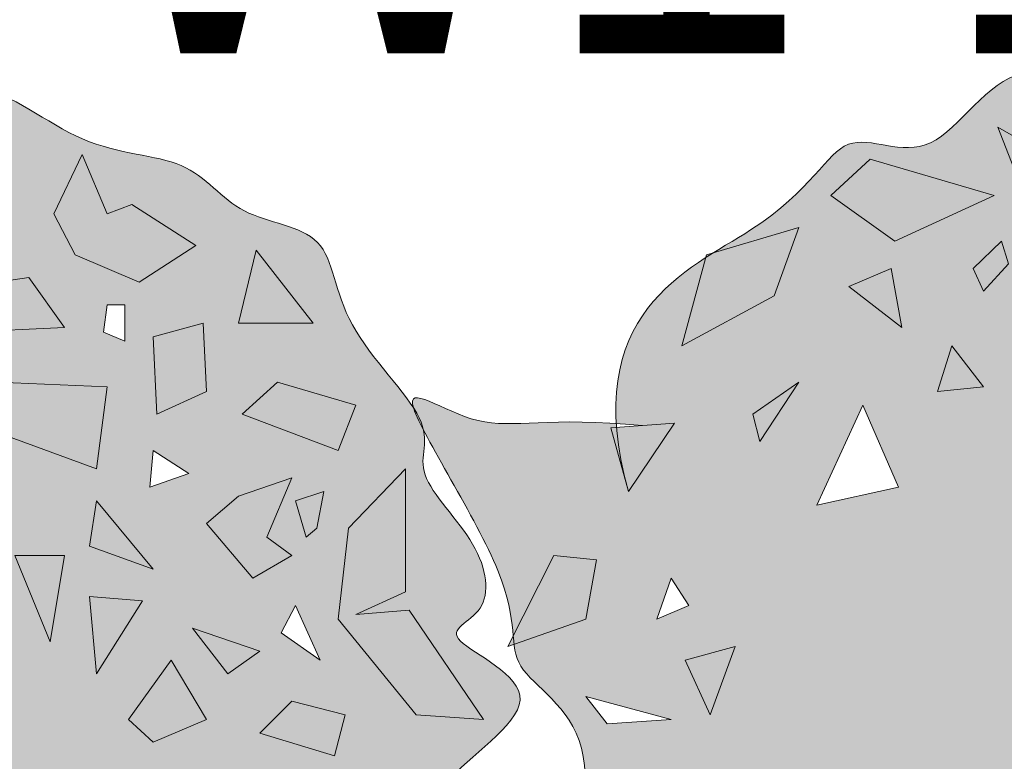
# Model space of a CAD drawing. Units: metres. Extents: x 4298.5 to 4325.2, y 2075 to 2095.8.
# Tile 7 of 35: x 4306.6693 to 4307.1445, y 2079.3365 to 2079.6943. Entities that reach past the tile are written whole.
import ezdxf

# ---------------------------------------------------------------- set-up
doc = ezdxf.new("R2010")
doc.units = ezdxf.units.M
doc.layers.add('A-ANNO-DIMS', color=2, linetype='Continuous', lineweight=18)
doc.layers.add('L-PLNT', color=94, linetype='Continuous', lineweight=13)
doc.layers.add('L-PLNT-PATT', color=116, linetype='Continuous', lineweight=13, true_color=0x13823e)
doc.styles.get("Standard").update_dxf_attribs({"font": 'arial.ttf'})
doc.dimstyles.get("Standard").update_dxf_attribs({"dimtxt": 0.18, "dimasz": 0.18, "dimexe": 0.18, "dimexo": 0.0625, "dimgap": 0.09, "dimtad": 0, "dimtih": 1, "dimtoh": 1, "dimdec": 4, "dimzin": 0, "dimdsep": 46, "dimtxsty": 'Standard', "dimcen": 0.09, "dimadec": 0, "dimazin": 0, "dimtfac": 1, "dimtdec": 4, "dimtofl": 0, "dimtmove": 0, "dimatfit": 3, "dimfxl": 1, "dimtolj": 1, "dimtzin": 0, "dimarcsym": 0})

# ---------------------------------------------------------------- blocks, each defined once
blk = doc.blocks.new('*U9')
for points in [[(-2.003, 11.656), (-1.598, 10.618), (-0.518, 10.099), (-0.181, 10.618), (-0.788, 10.964)], [(-4.432, 11.051), (-5.175, 10.359), (-3.96, 9.493), (-2.07, 10.359)], [(4.139, 11.137), (3.599, 10.013), (4.004, 9.234), (5.218, 8.715), (6.298, 9.407), (5.083, 10.186), (4.611, 10.013)], [(-5.782, 9.753), (-7.537, 9.234), (-8.009, 7.504), (-6.255, 8.455)], [(-1.935, 9.493), (-2.475, 8.974), (-2.273, 8.542), (-1.8, 9.061)], [(7.446, 9.32), (7.108, 7.936), (8.525, 7.936)], [(-4.837, 8.628), (-3.825, 7.85), (-4.027, 8.974)], [(1.372, 8.542), (3.126, 8.801), (3.801, 7.85), (1.912, 7.763)], [(4.611, 8.282), (4.544, 7.763), (4.949, 7.59), (4.949, 8.282)], [(6.433, 7.936), (5.488, 7.676), (5.556, 6.206), (6.501, 6.638)], [(-2.88, 7.504), (-3.15, 6.638), (-2.273, 6.725)], [(-5.782, 6.811), (-6.659, 6.206), (-6.524, 5.687)], [(2.519, 6.811), (2.519, 5.86), (4.409, 5.167), (4.611, 6.725)], [(7.851, 6.811), (7.176, 6.206), (8.998, 5.514), (9.335, 6.379)], [(-4.567, 6.379), (-5.445, 4.475), (-3.892, 4.821)], [(-8.144, 6.033), (-9.359, 5.946), (-9.022, 4.735)], [(5.488, 5.514), (5.421, 4.821), (6.163, 5.081)], [(10.28, 5.167), (9.2, 4.043), (8.998, 2.312), (10.482, 0.495), (11.765, 0.409), (10.348, 2.485), (9.335, 2.399), (10.28, 2.831)], [(8.12, 4.994), (7.108, 4.648), (6.501, 4.129), (7.378, 3.091), (8.12, 3.524), (7.648, 3.87)], [(8.728, 4.735), (8.188, 4.562), (8.39, 3.87), (8.593, 4.043)], [(4.409, 4.562), (4.274, 3.697), (5.488, 3.264)], [(-11.316, 1.793), (-9.831, 2.312), (-9.629, 3.437), (-10.439, 3.524)], [(3.531, 1.88), (2.856, 3.524), (3.801, 3.524)], [(-8.212, 3.091), (-8.482, 2.312), (-7.874, 2.572)], [(4.274, 2.745), (5.286, 2.658), (4.409, 1.274)], [(8.188, 2.572), (7.918, 2.053), (8.66, 1.534)], [(7.513, 1.707), (6.906, 1.274), (6.231, 2.139)], [(-6.997, 1.793), (-7.942, 1.534), (-7.469, 0.495)], [(5.826, 1.534), (5.016, 0.409), (5.488, -0.024), (6.501, 0.409)], [(-8.212, 0.409), (-9.426, 0.322), (-9.831, 0.841)], [(8.12, 0.755), (7.513, 0.149), (8.93, -0.283), (9.133, 0.495)]]:
    blk.add_lwpolyline(points, close=True)
blk = doc.blocks.new('*D23')
at = {"layer": 'A-ANNO-DIMS', "color": 0, "lineweight": -2, "transparency": 16777216}
for p, q in [((4308.16058, 2079.85556), (4308.16058, 2079.58806)), ((4309.16058, 2079.85556), (4309.16058, 2079.58806)), ((4308.16058, 2079.76806), (4307.98058, 2079.76806)), ((4308.98058, 2079.76806), (4308.34058, 2079.76806))]:
    blk.add_line(p, q, dxfattribs=at)
at = {"layer": 'A-ANNO-DIMS', "color": 0, "transparency": 16777216}
for points in [[(4308.34058, 2079.79806), (4308.34058, 2079.73806), (4308.16058, 2079.76806)], [(4308.98058, 2079.79806), (4308.98058, 2079.73806), (4309.16058, 2079.76806)]]:
    blk.add_solid(points, dxfattribs=at)
at = {"layer": 'Defpoints', "color": 0, "transparency": 16777216}
for p in [(4308.16058, 2079.91806), (4309.16058, 2079.91806), (4308.16058, 2079.76806)]:
    blk.add_point(p, dxfattribs=at)
at = {"layer": 'A-ANNO-DIMS', "color": 0, "transparency": 16777216, "insert": (4306.70861, 2079.76806), "char_height": 0.18, "attachment_point": 5}
blk.add_mtext('\\A1;WINDOW W1 1 TYP.', dxfattribs=at)
blk = doc.blocks.new('*D47')
at = {"layer": 'A-ANNO-DIMS', "color": 0, "lineweight": -2, "transparency": 16777216}
for p, q in [((4300.43058, 2084.49556), (4300.43058, 2074.98956)), ((4322.81058, 2084.49556), (4322.81058, 2074.98956)), ((4300.61058, 2075.16956), (4311.22515, 2075.16956)), ((4322.63058, 2075.16956), (4312.016, 2075.16956))]:
    blk.add_line(p, q, dxfattribs=at)
at = {"layer": 'A-ANNO-DIMS', "color": 0, "transparency": 16777216}
for points in [[(4300.61058, 2075.19956), (4300.61058, 2075.13956), (4300.43058, 2075.16956)], [(4322.63058, 2075.19956), (4322.63058, 2075.13956), (4322.81058, 2075.16956)]]:
    blk.add_solid(points, dxfattribs=at)
at = {"layer": 'Defpoints', "color": 0, "transparency": 16777216}
for p in [(4300.43058, 2084.55806), (4322.81058, 2084.55806), (4322.81058, 2075.16956)]:
    blk.add_point(p, dxfattribs=at)
at = {"layer": 'A-ANNO-DIMS', "color": 0, "transparency": 16777216, "insert": (4311.62058, 2075.16956), "char_height": 0.18, "attachment_point": 5}
blk.add_mtext('\\A1;22.38', dxfattribs=at)
blk = doc.blocks.new('*D54')
at = {"layer": 'A-ANNO-DIMS', "color": 0, "lineweight": -2, "transparency": 16777216}
for p, q in [((4305.59808, 2079.82806), (4299.09208, 2079.82806)), ((4299.27208, 2079.64806), (4299.27208, 2078.26002)), ((4299.27208, 2076.50806), (4299.27208, 2077.89609)), ((4309.09808, 2076.32806), (4299.09208, 2076.32806))]:
    blk.add_line(p, q, dxfattribs=at)
at = {"layer": 'A-ANNO-DIMS', "color": 0, "transparency": 16777216}
for points in [[(4299.24208, 2079.64806), (4299.30208, 2079.64806), (4299.27208, 2079.82806)], [(4299.24208, 2076.50806), (4299.30208, 2076.50806), (4299.27208, 2076.32806)]]:
    blk.add_solid(points, dxfattribs=at)
at = {"layer": 'Defpoints', "color": 0, "transparency": 16777216}
for p in [(4305.66058, 2079.82806), (4299.27208, 2076.32806), (4309.16058, 2076.32806)]:
    blk.add_point(p, dxfattribs=at)
at = {"layer": 'A-ANNO-DIMS', "color": 0, "transparency": 16777216, "insert": (4299.27208, 2078.07806), "char_height": 0.18, "attachment_point": 5}
blk.add_mtext('\\A1;3.5', dxfattribs=at)
blk = doc.blocks.new('*D59')
at = {"layer": 'A-ANNO-DIMS', "color": 0, "lineweight": -2, "transparency": 16777216}
for p, q in [((4305.89058, 2079.99556), (4305.89058, 2074.98956)), ((4307.39058, 2079.99556), (4307.39058, 2074.98956)), ((4306.07058, 2075.16956), (4306.39452, 2075.16956)), ((4307.21058, 2075.16956), (4306.88663, 2075.16956))]:
    blk.add_line(p, q, dxfattribs=at)
at = {"layer": 'A-ANNO-DIMS', "color": 0, "transparency": 16777216}
for points in [[(4306.07058, 2075.19956), (4306.07058, 2075.13956), (4305.89058, 2075.16956)], [(4307.21058, 2075.19956), (4307.21058, 2075.13956), (4307.39058, 2075.16956)]]:
    blk.add_solid(points, dxfattribs=at)
at = {"layer": 'Defpoints', "color": 0, "transparency": 16777216}
for p in [(4305.89058, 2080.05806), (4307.39058, 2080.05806), (4307.39058, 2075.16956)]:
    blk.add_point(p, dxfattribs=at)
at = {"layer": 'A-ANNO-DIMS', "color": 0, "transparency": 16777216, "insert": (4306.64058, 2075.16956), "char_height": 0.18, "attachment_point": 5}
blk.add_mtext('\\A1;1.5', dxfattribs=at)
blk = doc.blocks.new('*D78')
at = {"layer": 'A-ANNO-DIMS', "color": 0, "lineweight": -2, "transparency": 16777216}
for p, q in [((4312.4969, 2079.73934), (4312.4969, 2079.91934)), ((4312.4069, 2079.82934), (4312.5869, 2079.82934)), ((4305.38467, 2076.78063), (4307.88631, 2077.85298)), ((4305.20467, 2076.78063), (4305.38467, 2076.78063))]:
    blk.add_line(p, q, dxfattribs=at)
at = {"layer": 'A-ANNO-DIMS', "color": 0, "transparency": 16777216}
blk.add_solid([(4307.87449, 2077.88055), (4307.89813, 2077.8254), (4308.05176, 2077.92389)], dxfattribs=at)
at = {"layer": 'Defpoints', "color": 0, "transparency": 16777216}
for p in [(4312.4969, 2079.82934), (4308.05176, 2077.92389)]:
    blk.add_point(p, dxfattribs=at)
at = {"layer": 'A-ANNO-DIMS', "color": 0, "transparency": 16777216, "insert": (4304.52998, 2076.78063), "char_height": 0.18, "attachment_point": 5}
blk.add_mtext('\\A1;2X R4.836', dxfattribs=at)

msp = doc.modelspace()

# ---------------------------------------------------------------- hatches: boundary and pattern name
at = {"layer": 'L-PLNT-PATT'}
h = msp.add_hatch(color=256, dxfattribs=at)
h.dxf.hatch_style = 1
edge = h.paths.add_edge_path()
edge.add_spline(control_points=[(4306.69044, 2079.08578), (4306.69302, 2079.08709), (4306.71165, 2079.09641), (4306.74745, 2079.10618), (4306.80198, 2079.12944), (4306.83132, 2079.13707), (4306.8126, 2079.16551), (4306.86518, 2079.18971), (4306.83145, 2079.21603), (4306.85847, 2079.27577), (4306.8772, 2079.29524), (4306.86058, 2079.32373), (4306.93479, 2079.3686), (4306.86486, 2079.39817), (4306.89754, 2079.40581), (4306.89356, 2079.44094), (4306.85545, 2079.47755), (4306.87404, 2079.4969), (4306.82098, 2079.54789), (4306.82098, 2079.59392), (4306.77312, 2079.5973), (4306.75268, 2079.62919), (4306.69947, 2079.62919), (4306.64714, 2079.67454), (4306.61235, 2079.63742), (4306.55167, 2079.68828), (4306.51176, 2079.61822), (4306.46721, 2079.64819), (4306.45286, 2079.60881), (4306.41256, 2079.5858), (4306.40621, 2079.58183)], knot_values=[0.818571, 0.818571, 0.818571, 0.818571, 0.97924, 1.97924, 2.97924, 3.97924, 4.97924, 5.97924, 6.97924, 7.97924, 8.97924, 9.97924, 10.97924, 11.97924, 12.97924, 13.97924, 14.97924, 15.97924, 16.97924, 17.97924, 18.97924, 19.97924, 20.97924, 21.97924, 22.97924, 23.97924, 24.97924, 25.97924, 26.97924, 27.16067, 27.16067, 27.16067, 27.16067], degree=3, periodic=0)
edge.add_line((4306.40621, 2079.58183), (4306.44747, 2079.59404))
edge.add_line((4306.44747, 2079.59404), (4306.43546, 2079.56107))
edge.add_line((4306.43546, 2079.56107), (4306.39091, 2079.53691))
edge.add_line((4306.39091, 2079.53691), (4306.40253, 2079.5795))
edge.add_spline(control_points=[(4306.40253, 2079.5795), (4306.37988, 2079.56484), (4306.35659, 2079.5439), (4306.35932, 2079.49949)], knot_values=[0.141368, 0.141368, 0.141368, 0.141368, 0.783694, 0.783694, 0.783694, 0.783694], degree=3, periodic=0)
edge.add_spline(control_points=[(4306.35932, 2079.49949), (4306.36329, 2079.49923), (4306.36753, 2079.49889), (4306.37205, 2079.49844)], knot_values=[40.901028, 40.901028, 40.901028, 40.901028, 41, 41, 41, 41], degree=3, periodic=0)
edge.add_line((4306.37205, 2079.49844), (4306.38748, 2079.49955))
edge.add_line((4306.38748, 2079.49955), (4306.36518, 2079.46658))
edge.add_line((4306.36518, 2079.46658), (4306.35662, 2079.49734))
edge.add_line((4306.35662, 2079.49734), (4306.35944, 2079.49754))
edge.add_spline(control_points=[(4306.35945, 2079.49754), (4306.3594, 2079.4982), (4306.35936, 2079.49885), (4306.35932, 2079.49949)], knot_values=[0.13204, 0.13204, 0.13204, 0.13204, 0.141368, 0.141368, 0.141368, 0.141368], degree=3, periodic=0)
edge.add_spline(control_points=[(4306.35932, 2079.49949), (4306.3231, 2079.50184), (4306.2915, 2079.49199), (4306.23947, 2079.53397), (4306.30655, 2079.43142), (4306.30887, 2079.40456), (4306.30956, 2079.39708)], knot_values=[37.439141, 37.439141, 37.439141, 37.439141, 38.340169, 39.340169, 40.340169, 40.901028, 40.901028, 40.901028, 40.901028], degree=3, periodic=0)
edge.add_line((4306.30956, 2079.39708), (4306.32919, 2079.43582))
edge.add_line((4306.32919, 2079.43582), (4306.34976, 2079.43361))
edge.add_line((4306.34976, 2079.43361), (4306.34463, 2079.40504))
edge.add_line((4306.34463, 2079.40504), (4306.30999, 2079.39293))
edge.add_spline(control_points=[(4306.30999, 2079.39293), (4306.31047, 2079.38899), (4306.31356, 2079.37544), (4306.35492, 2079.35449), (4306.33345, 2079.25721), (4306.3657, 2079.23836), (4306.43192, 2079.23836), (4306.45469, 2079.18462), (4306.45818, 2079.14915), (4306.53918, 2079.08309), (4306.59748, 2079.09986), (4306.64786, 2079.06298), (4306.677, 2079.07895), (4306.69044, 2079.08578)], knot_values=[27.16067, 27.16067, 27.16067, 27.16067, 27.490087, 28.490087, 29.490087, 30.490087, 31.490087, 32.490087, 33.490087, 34.490087, 35.490087, 36.490087, 37.329418, 37.329418, 37.329418, 37.329418], degree=3, periodic=0)
edge.add_line((4306.69044, 2079.08578), (4306.68402, 2079.09297))
edge.add_line((4306.68402, 2079.09297), (4306.69774, 2079.10618))
edge.add_line((4306.69774, 2079.10618), (4306.71147, 2079.09517))
h.paths.add_polyline_path([(4306.66688, 2079.43582), (4306.69088, 2079.43582), (4306.68402, 2079.39406)], flags=16)
h.paths.add_polyline_path([(4306.7029, 2079.41603), (4306.7286, 2079.41382), (4306.70633, 2079.37867)], flags=16)
h.paths.add_polyline_path([(4306.49548, 2079.46876), (4306.45603, 2079.45998), (4306.47834, 2079.50834)], flags=16)
h.paths.add_polyline_path([(4306.62233, 2079.49734), (4306.5966, 2079.51052), (4306.61374, 2079.5281)], flags=16)
h.paths.add_polyline_path([(4306.7029, 2079.44022), (4306.70633, 2079.46219), (4306.73373, 2079.42922)], flags=16)
h.paths.add_polyline_path([(4306.72174, 2079.3567), (4306.74232, 2079.38527), (4306.75946, 2079.3567), (4306.73373, 2079.3457)], flags=16)
h.paths.add_polyline_path([(4306.65832, 2079.49516), (4306.65832, 2079.51931), (4306.71146, 2079.51713), (4306.70633, 2079.47755)], flags=16)
h.paths.add_polyline_path([(4306.63775, 2079.50613), (4306.63775, 2079.52591), (4306.66175, 2079.53691), (4306.64803, 2079.52152)], flags=16)
h.paths.add_polyline_path([(4306.5366, 2079.51713), (4306.51433, 2079.51492), (4306.52118, 2079.53691)], flags=16)
h.paths.add_polyline_path([(4306.55032, 2079.5281), (4306.56061, 2079.56328), (4306.5949, 2079.57646), (4306.60175, 2079.54349)], flags=16)
h.paths.add_polyline_path([(4306.41661, 2079.39185), (4306.40462, 2079.35888), (4306.39261, 2079.38527)], flags=16)
h.paths.add_polyline_path([(4306.7526, 2079.40064), (4306.78517, 2079.38967), (4306.76975, 2079.37867)], flags=16)
h.paths.add_polyline_path([(4306.73203, 2079.46876), (4306.73373, 2079.48637), (4306.75088, 2079.47537)], flags=16)
h.paths.add_polyline_path([(4306.6429, 2079.54349), (4306.62919, 2079.56328), (4306.67374, 2079.56986), (4306.69088, 2079.5457)], flags=16)
h.paths.add_polyline_path([(4306.75774, 2079.32812), (4306.79203, 2079.32592), (4306.75774, 2079.30834)], flags=16)
h.paths.add_polyline_path([(4306.39434, 2079.41164), (4306.37889, 2079.40504), (4306.38575, 2079.42482)], flags=16)
h.paths.add_polyline_path([(4306.49718, 2079.5457), (4306.47148, 2079.56546), (4306.49205, 2079.57425)], flags=16)
h.paths.add_polyline_path([(4306.42863, 2079.49076), (4306.4252, 2079.50394), (4306.44747, 2079.51931)], flags=16)
h.paths.add_polyline_path([(4306.5366, 2079.56328), (4306.53147, 2079.57425), (4306.54519, 2079.58743), (4306.54862, 2079.57646)], flags=16)
h.paths.add_polyline_path([(4306.75946, 2079.45119), (4306.77488, 2079.46437), (4306.80058, 2079.47316), (4306.7886, 2079.44461), (4306.80058, 2079.43582), (4306.78174, 2079.42482)], flags=16)
h.paths.add_polyline_path([(4306.38575, 2079.3567), (4306.35492, 2079.35449), (4306.34463, 2079.36767)], flags=16)
h.paths.add_polyline_path([(4306.73546, 2079.50394), (4306.73373, 2079.54128), (4306.75774, 2079.54789), (4306.75946, 2079.51492)], flags=16)
h.paths.add_polyline_path([(4306.78517, 2079.3501), (4306.80058, 2079.36549), (4306.82632, 2079.35888), (4306.82116, 2079.33912)], flags=16)
h.paths.add_polyline_path([(4306.70975, 2079.54349), (4306.71146, 2079.55667), (4306.72004, 2079.55667), (4306.72004, 2079.5391)], flags=16)
h.paths.add_polyline_path([(4306.63604, 2079.58085), (4306.64117, 2079.59404), (4306.66002, 2079.59843), (4306.65316, 2079.58525)], flags=16)
h.paths.add_polyline_path([(4306.79545, 2079.39846), (4306.80231, 2079.41164), (4306.8143, 2079.38527)], flags=16)
h.paths.add_polyline_path([(4306.78689, 2079.29297), (4306.80574, 2079.30176), (4306.79716, 2079.28197)], flags=16)
h.paths.add_polyline_path([(4306.58118, 2079.60283), (4306.55375, 2079.61601), (4306.54346, 2079.64237), (4306.57432, 2079.6248), (4306.58974, 2079.61601)], flags=16)
h.paths.add_polyline_path([(4306.61374, 2079.60064), (4306.60861, 2079.63359), (4306.62576, 2079.65119), (4306.65832, 2079.62701)], flags=16)
h.paths.add_polyline_path([(4306.49375, 2079.58743), (4306.46289, 2079.60943), (4306.48176, 2079.62701), (4306.54176, 2079.60943)], flags=16)
h.paths.add_polyline_path([(4306.77661, 2079.50394), (4306.79375, 2079.51931), (4306.83145, 2079.50834), (4306.82289, 2079.48637)], flags=16)
h.paths.add_polyline_path([(4306.69604, 2079.58085), (4306.68575, 2079.60064), (4306.69947, 2079.62919), (4306.71146, 2079.60064), (4306.72345, 2079.60504), (4306.75431, 2079.58525), (4306.72687, 2079.56767)], flags=16)
h.paths.add_polyline_path([(4306.80744, 2079.44461), (4306.80231, 2079.46219), (4306.81603, 2079.46658), (4306.8126, 2079.449)], flags=16)
h.paths.add_polyline_path([(4306.82289, 2079.40504), (4306.82802, 2079.449), (4306.85545, 2079.47755), (4306.85545, 2079.41822), (4306.83145, 2079.40725), (4306.85718, 2079.40943), (4306.89317, 2079.3567), (4306.86058, 2079.35888)], flags=16)
h.paths.add_polyline_path([(4306.56233, 2079.13034), (4306.56919, 2079.10397), (4306.5349, 2079.11276)], flags=16)
h.paths.add_polyline_path([(4306.77488, 2079.54789), (4306.78347, 2079.58304), (4306.81087, 2079.54789)], flags=16)
h.paths.add_polyline_path([(4306.83145, 2079.30176), (4306.85202, 2079.28197), (4306.8366, 2079.25121)], flags=16)
h.paths.add_polyline_path([(4306.84173, 2079.31273), (4306.85032, 2079.33033), (4306.86058, 2079.32373)], flags=16)
h.paths.add_polyline_path([(4306.71146, 2079.13912), (4306.7286, 2079.14352), (4306.72174, 2079.11936)], flags=16)
h.paths.add_polyline_path([(4306.79716, 2079.21385), (4306.83145, 2079.21603), (4306.80917, 2079.18749)], flags=16)
h.paths.add_polyline_path([(4306.75088, 2079.1633), (4306.76975, 2079.17649), (4306.77831, 2079.15891), (4306.74918, 2079.11936)], flags=16)
h.paths.add_polyline_path([(4306.79545, 2079.15452), (4306.8126, 2079.16551), (4306.79888, 2079.14133)], flags=16)
h = msp.add_hatch(color=256, dxfattribs=at)
h.dxf.hatch_style = 1
edge = h.paths.add_edge_path()
edge.add_spline(control_points=[(4307.28832, 2079.08578), (4307.29089, 2079.08709), (4307.30952, 2079.09641), (4307.34532, 2079.10618), (4307.39985, 2079.12944), (4307.4292, 2079.13707), (4307.41047, 2079.16551), (4307.46306, 2079.18971), (4307.42932, 2079.21603), (4307.45635, 2079.27577), (4307.47508, 2079.29524), (4307.45845, 2079.32373), (4307.53267, 2079.3686), (4307.46273, 2079.39817), (4307.49542, 2079.40581), (4307.49143, 2079.44094), (4307.45332, 2079.47755), (4307.47191, 2079.4969), (4307.41885, 2079.54789), (4307.41885, 2079.59392), (4307.37099, 2079.5973), (4307.35056, 2079.62919), (4307.29734, 2079.62919), (4307.24502, 2079.67454), (4307.21022, 2079.63742), (4307.14954, 2079.68828), (4307.10964, 2079.61822), (4307.06508, 2079.64819), (4307.05073, 2079.60881), (4307.01044, 2079.5858), (4307.00408, 2079.58183)], knot_values=[0.818571, 0.818571, 0.818571, 0.818571, 0.97924, 1.97924, 2.97924, 3.97924, 4.97924, 5.97924, 6.97924, 7.97924, 8.97924, 9.97924, 10.97924, 11.97924, 12.97924, 13.97924, 14.97924, 15.97924, 16.97924, 17.97924, 18.97924, 19.97924, 20.97924, 21.97924, 22.97924, 23.97924, 24.97924, 25.97924, 26.97924, 27.16067, 27.16067, 27.16067, 27.16067], degree=3, periodic=0)
edge.add_line((4307.00408, 2079.58183), (4307.04535, 2079.59404))
edge.add_line((4307.04535, 2079.59404), (4307.03333, 2079.56107))
edge.add_line((4307.03333, 2079.56107), (4306.98878, 2079.53691))
edge.add_line((4306.98878, 2079.53691), (4307.0004, 2079.5795))
edge.add_spline(control_points=[(4307.0004, 2079.5795), (4306.97776, 2079.56484), (4306.95447, 2079.5439), (4306.95719, 2079.49949)], knot_values=[0.141368, 0.141368, 0.141368, 0.141368, 0.783694, 0.783694, 0.783694, 0.783694], degree=3, periodic=0)
edge.add_spline(control_points=[(4306.95719, 2079.49949), (4306.96117, 2079.49923), (4306.9654, 2079.49889), (4306.96992, 2079.49844)], knot_values=[40.901028, 40.901028, 40.901028, 40.901028, 41, 41, 41, 41], degree=3, periodic=0)
edge.add_line((4306.96992, 2079.49844), (4306.98535, 2079.49955))
edge.add_line((4306.98535, 2079.49955), (4306.96305, 2079.46658))
edge.add_line((4306.96305, 2079.46658), (4306.95449, 2079.49734))
edge.add_line((4306.95449, 2079.49734), (4306.95732, 2079.49754))
edge.add_spline(control_points=[(4306.95733, 2079.49754), (4306.95728, 2079.4982), (4306.95723, 2079.49885), (4306.95719, 2079.49949)], knot_values=[0.13204, 0.13204, 0.13204, 0.13204, 0.141368, 0.141368, 0.141368, 0.141368], degree=3, periodic=0)
edge.add_spline(control_points=[(4306.95719, 2079.49949), (4306.92097, 2079.50184), (4306.88937, 2079.49199), (4306.83734, 2079.53397), (4306.90442, 2079.43142), (4306.90674, 2079.40456), (4306.90744, 2079.39708)], knot_values=[37.439141, 37.439141, 37.439141, 37.439141, 38.340169, 39.340169, 40.340169, 40.901028, 40.901028, 40.901028, 40.901028], degree=3, periodic=0)
edge.add_line((4306.90744, 2079.39708), (4306.92706, 2079.43582))
edge.add_line((4306.92706, 2079.43582), (4306.94764, 2079.43361))
edge.add_line((4306.94764, 2079.43361), (4306.9425, 2079.40504))
edge.add_line((4306.9425, 2079.40504), (4306.90786, 2079.39293))
edge.add_spline(control_points=[(4306.90786, 2079.39293), (4306.90835, 2079.38899), (4306.91143, 2079.37544), (4306.95279, 2079.35449), (4306.93133, 2079.25721), (4306.96358, 2079.23836), (4307.0298, 2079.23836), (4307.05256, 2079.18462), (4307.05606, 2079.14915), (4307.13706, 2079.08309), (4307.19535, 2079.09986), (4307.24573, 2079.06298), (4307.27487, 2079.07895), (4307.28832, 2079.08578)], knot_values=[27.16067, 27.16067, 27.16067, 27.16067, 27.490087, 28.490087, 29.490087, 30.490087, 31.490087, 32.490087, 33.490087, 34.490087, 35.490087, 36.490087, 37.329418, 37.329418, 37.329418, 37.329418], degree=3, periodic=0)
edge.add_line((4307.28832, 2079.08578), (4307.2819, 2079.09297))
edge.add_line((4307.2819, 2079.09297), (4307.29562, 2079.10618))
edge.add_line((4307.29562, 2079.10618), (4307.30934, 2079.09517))
h.paths.add_polyline_path([(4307.26475, 2079.43582), (4307.28876, 2079.43582), (4307.2819, 2079.39406)], flags=16)
h.paths.add_polyline_path([(4307.30077, 2079.41603), (4307.32648, 2079.41382), (4307.3042, 2079.37867)], flags=16)
h.paths.add_polyline_path([(4307.09335, 2079.46876), (4307.05391, 2079.45998), (4307.07621, 2079.50834)], flags=16)
h.paths.add_polyline_path([(4307.2202, 2079.49734), (4307.19447, 2079.51052), (4307.21162, 2079.5281)], flags=16)
h.paths.add_polyline_path([(4307.30077, 2079.44022), (4307.3042, 2079.46219), (4307.33161, 2079.42922)], flags=16)
h.paths.add_polyline_path([(4307.31962, 2079.3567), (4307.34019, 2079.38527), (4307.35734, 2079.3567), (4307.33161, 2079.3457)], flags=16)
h.paths.add_polyline_path([(4307.25619, 2079.49516), (4307.25619, 2079.51931), (4307.30933, 2079.51713), (4307.3042, 2079.47755)], flags=16)
h.paths.add_polyline_path([(4307.23562, 2079.50613), (4307.23562, 2079.52591), (4307.25962, 2079.53691), (4307.24591, 2079.52152)], flags=16)
h.paths.add_polyline_path([(4307.13448, 2079.51713), (4307.1122, 2079.51492), (4307.11906, 2079.53691)], flags=16)
h.paths.add_polyline_path([(4307.14819, 2079.5281), (4307.15848, 2079.56328), (4307.19277, 2079.57646), (4307.19963, 2079.54349)], flags=16)
h.paths.add_polyline_path([(4307.01449, 2079.39185), (4307.0025, 2079.35888), (4306.99048, 2079.38527)], flags=16)
h.paths.add_polyline_path([(4307.35048, 2079.40064), (4307.38304, 2079.38967), (4307.36762, 2079.37867)], flags=16)
h.paths.add_polyline_path([(4307.32991, 2079.46876), (4307.33161, 2079.48637), (4307.34875, 2079.47537)], flags=16)
h.paths.add_polyline_path([(4307.24078, 2079.54349), (4307.22706, 2079.56328), (4307.27161, 2079.56986), (4307.28876, 2079.5457)], flags=16)
h.paths.add_polyline_path([(4307.35561, 2079.32812), (4307.3899, 2079.32592), (4307.35561, 2079.30834)], flags=16)
h.paths.add_polyline_path([(4306.99221, 2079.41164), (4306.97677, 2079.40504), (4306.98363, 2079.42482)], flags=16)
h.paths.add_polyline_path([(4307.09506, 2079.5457), (4307.06935, 2079.56546), (4307.08993, 2079.57425)], flags=16)
h.paths.add_polyline_path([(4307.0265, 2079.49076), (4307.02307, 2079.50394), (4307.04535, 2079.51931)], flags=16)
h.paths.add_polyline_path([(4307.13448, 2079.56328), (4307.12935, 2079.57425), (4307.14306, 2079.58743), (4307.14649, 2079.57646)], flags=16)
h.paths.add_polyline_path([(4307.35734, 2079.45119), (4307.37275, 2079.46437), (4307.39846, 2079.47316), (4307.38647, 2079.44461), (4307.39846, 2079.43582), (4307.37961, 2079.42482)], flags=16)
h.paths.add_polyline_path([(4306.98363, 2079.3567), (4306.95279, 2079.35449), (4306.9425, 2079.36767)], flags=16)
h.paths.add_polyline_path([(4307.33333, 2079.50394), (4307.33161, 2079.54128), (4307.35561, 2079.54789), (4307.35734, 2079.51492)], flags=16)
h.paths.add_polyline_path([(4307.38304, 2079.3501), (4307.39846, 2079.36549), (4307.42419, 2079.35888), (4307.41903, 2079.33912)], flags=16)
h.paths.add_polyline_path([(4307.30763, 2079.54349), (4307.30933, 2079.55667), (4307.31792, 2079.55667), (4307.31792, 2079.5391)], flags=16)
h.paths.add_polyline_path([(4307.23392, 2079.58085), (4307.23905, 2079.59404), (4307.2579, 2079.59843), (4307.25104, 2079.58525)], flags=16)
h.paths.add_polyline_path([(4307.39333, 2079.39846), (4307.40019, 2079.41164), (4307.41218, 2079.38527)], flags=16)
h.paths.add_polyline_path([(4307.38477, 2079.29297), (4307.40362, 2079.30176), (4307.39503, 2079.28197)], flags=16)
h.paths.add_polyline_path([(4307.17905, 2079.60283), (4307.15162, 2079.61601), (4307.14134, 2079.64237), (4307.1722, 2079.6248), (4307.18761, 2079.61601)], flags=16)
h.paths.add_polyline_path([(4307.21162, 2079.60064), (4307.20649, 2079.63359), (4307.22363, 2079.65119), (4307.25619, 2079.62701)], flags=16)
h.paths.add_polyline_path([(4307.09163, 2079.58743), (4307.06077, 2079.60943), (4307.07964, 2079.62701), (4307.13963, 2079.60943)], flags=16)
h.paths.add_polyline_path([(4307.37448, 2079.50394), (4307.39163, 2079.51931), (4307.42932, 2079.50834), (4307.42076, 2079.48637)], flags=16)
h.paths.add_polyline_path([(4307.29391, 2079.58085), (4307.28363, 2079.60064), (4307.29734, 2079.62919), (4307.30933, 2079.60064), (4307.32132, 2079.60504), (4307.35218, 2079.58525), (4307.32475, 2079.56767)], flags=16)
h.paths.add_polyline_path([(4307.40532, 2079.44461), (4307.40019, 2079.46219), (4307.4139, 2079.46658), (4307.41047, 2079.449)], flags=16)
h.paths.add_polyline_path([(4307.42076, 2079.40504), (4307.42589, 2079.449), (4307.45332, 2079.47755), (4307.45332, 2079.41822), (4307.42932, 2079.40725), (4307.45505, 2079.40943), (4307.49104, 2079.3567), (4307.45845, 2079.35888)], flags=16)
h.paths.add_polyline_path([(4307.16021, 2079.13034), (4307.16707, 2079.10397), (4307.13278, 2079.11276)], flags=16)
h.paths.add_polyline_path([(4307.37275, 2079.54789), (4307.38134, 2079.58304), (4307.40875, 2079.54789)], flags=16)
h.paths.add_polyline_path([(4307.42932, 2079.30176), (4307.44989, 2079.28197), (4307.43448, 2079.25121)], flags=16)
h.paths.add_polyline_path([(4307.43961, 2079.31273), (4307.44819, 2079.33033), (4307.45845, 2079.32373)], flags=16)
h.paths.add_polyline_path([(4307.30933, 2079.13912), (4307.32648, 2079.14352), (4307.31962, 2079.11936)], flags=16)
h.paths.add_polyline_path([(4307.39503, 2079.21385), (4307.42932, 2079.21603), (4307.40704, 2079.18749)], flags=16)
h.paths.add_polyline_path([(4307.34875, 2079.1633), (4307.36762, 2079.17649), (4307.37618, 2079.15891), (4307.34705, 2079.11936)], flags=16)
h.paths.add_polyline_path([(4307.39333, 2079.15452), (4307.41047, 2079.16551), (4307.39676, 2079.14133)], flags=16)
h = msp.add_hatch(color=256, dxfattribs=at)
h.dxf.hatch_style = 1
h.paths.add_polyline_path([(4306.70633, 2079.47755), (4306.71146, 2079.51713), (4306.65832, 2079.51931), (4306.65832, 2079.49516)])
h.paths.add_polyline_path([(4306.7526, 2079.40064), (4306.76975, 2079.37867), (4306.78517, 2079.38967)])
h.paths.add_polyline_path([(4306.73373, 2079.54128), (4306.73546, 2079.50394), (4306.75946, 2079.51492), (4306.75774, 2079.54789)])
h.paths.add_polyline_path([(4306.75431, 2079.58525), (4306.72345, 2079.60504), (4306.71146, 2079.60064), (4306.69947, 2079.62919), (4306.68575, 2079.60064), (4306.69604, 2079.58085), (4306.72687, 2079.56767)])
h.paths.add_polyline_path([(4306.60003, 2079.0776), (4306.61547, 2079.06), (4306.66002, 2079.05782)])
h.paths.add_polyline_path([(4306.58118, 2079.60283), (4306.58974, 2079.61601), (4306.57432, 2079.6248), (4306.54346, 2079.64237), (4306.55375, 2079.61601)])
h.paths.add_polyline_path([(4306.48176, 2079.62701), (4306.46289, 2079.60943), (4306.49375, 2079.58743), (4306.54176, 2079.60943)])
h.paths.add_polyline_path([(4306.56061, 2079.56328), (4306.55032, 2079.5281), (4306.60175, 2079.54349), (4306.5949, 2079.57646)])
h.paths.add_polyline_path([(4306.54862, 2079.57646), (4306.54519, 2079.58743), (4306.53147, 2079.57425), (4306.5366, 2079.56328)])
h.paths.add_polyline_path([(4306.52118, 2079.53691), (4306.51433, 2079.51492), (4306.5366, 2079.51713)])
h.paths.add_polyline_path([(4306.49718, 2079.5457), (4306.49205, 2079.57425), (4306.47148, 2079.56546)])
h.paths.add_polyline_path([(4306.4029, 2079.58085), (4306.39091, 2079.53691), (4306.43546, 2079.56107), (4306.44747, 2079.59404)])
h.paths.add_polyline_path([(4306.44747, 2079.51931), (4306.4252, 2079.50394), (4306.42863, 2079.49076)])
h.paths.add_polyline_path([(4306.35662, 2079.49734), (4306.36518, 2079.46658), (4306.38748, 2079.49955)])
h.paths.add_polyline_path([(4306.30691, 2079.39185), (4306.34463, 2079.40504), (4306.34976, 2079.43361), (4306.32919, 2079.43582)])
h.paths.add_polyline_path([(4306.41661, 2079.39185), (4306.39261, 2079.38527), (4306.40462, 2079.35888)])
h.paths.add_polyline_path([(4306.3429, 2079.25779), (4306.33947, 2079.27758), (4306.32406, 2079.26219), (4306.32919, 2079.23364)])
h.paths.add_polyline_path([(4306.42177, 2079.21164), (4306.38405, 2079.20067), (4306.41661, 2079.18088)])
h.paths.add_polyline_path([(4306.44232, 2079.09737), (4306.48176, 2079.10618), (4306.47148, 2079.12155)])
h.paths.add_polyline_path([(4306.56233, 2079.13034), (4306.5349, 2079.11276), (4306.56919, 2079.10397)])
h.paths.add_polyline_path([(4306.69774, 2079.10618), (4306.68402, 2079.09297), (4306.69774, 2079.0776), (4306.71146, 2079.09518)])
h.paths.add_polyline_path([(4306.77831, 2079.15891), (4306.76975, 2079.17649), (4306.75088, 2079.1633), (4306.74918, 2079.11936)])
h.paths.add_polyline_path([(4306.74745, 2079.10618), (4306.73203, 2079.09297), (4306.75088, 2079.08858)])
h.paths.add_polyline_path([(4306.79545, 2079.15452), (4306.79888, 2079.14133), (4306.8126, 2079.16551)])
h.paths.add_polyline_path([(4306.8366, 2079.25121), (4306.85202, 2079.28197), (4306.83145, 2079.30176)])
h.paths.add_polyline_path([(4306.72174, 2079.3567), (4306.73373, 2079.3457), (4306.75946, 2079.3567), (4306.74232, 2079.38527)])
h.paths.add_polyline_path([(4306.86058, 2079.35888), (4306.89317, 2079.3567), (4306.85718, 2079.40943), (4306.83145, 2079.40725), (4306.85545, 2079.41822), (4306.85545, 2079.47755), (4306.82802, 2079.449), (4306.82289, 2079.40504)])
h.paths.add_polyline_path([(4306.80058, 2079.36549), (4306.78517, 2079.3501), (4306.82116, 2079.33912), (4306.82632, 2079.35888)])
h.paths.add_polyline_path([(4306.86058, 2079.32373), (4306.85032, 2079.33033), (4306.84173, 2079.31273)])
h.paths.add_polyline_path([(4306.80058, 2079.47316), (4306.77488, 2079.46437), (4306.75946, 2079.45119), (4306.78174, 2079.42482), (4306.80058, 2079.43582), (4306.7886, 2079.44461)])
h.paths.add_polyline_path([(4306.80231, 2079.46219), (4306.80744, 2079.44461), (4306.8126, 2079.449), (4306.81603, 2079.46658)])
h.paths.add_polyline_path([(4306.82289, 2079.48637), (4306.83145, 2079.50834), (4306.79375, 2079.51931), (4306.77661, 2079.50394)])
h.paths.add_polyline_path([(4306.73373, 2079.42922), (4306.70633, 2079.46219), (4306.7029, 2079.44022)])
h.paths.add_polyline_path([(4306.69088, 2079.43582), (4306.66688, 2079.43582), (4306.68402, 2079.39406)])
h.paths.add_polyline_path([(4306.7286, 2079.41382), (4306.7029, 2079.41603), (4306.70633, 2079.37867)])
h.paths.add_polyline_path([(4306.69088, 2079.5457), (4306.67374, 2079.56986), (4306.62919, 2079.56328), (4306.6429, 2079.54349)])
h.paths.add_polyline_path([(4306.64803, 2079.52152), (4306.66175, 2079.53691), (4306.63775, 2079.52591), (4306.63775, 2079.50613)])
h.paths.add_polyline_path([(4306.61374, 2079.5281), (4306.5966, 2079.51052), (4306.62233, 2079.49734)])
h.paths.add_polyline_path([(4306.65316, 2079.58525), (4306.66002, 2079.59843), (4306.64117, 2079.59404), (4306.63604, 2079.58085)])
h.paths.add_polyline_path([(4306.78347, 2079.58304), (4306.77488, 2079.54789), (4306.81087, 2079.54789)])
h = msp.add_hatch(color=256, dxfattribs=at)
h.dxf.hatch_style = 1
h.paths.add_polyline_path([(4307.3042, 2079.47755), (4307.30933, 2079.51713), (4307.25619, 2079.51931), (4307.25619, 2079.49516)])
h.paths.add_polyline_path([(4307.35048, 2079.40064), (4307.36762, 2079.37867), (4307.38304, 2079.38967)])
h.paths.add_polyline_path([(4307.33161, 2079.54128), (4307.33333, 2079.50394), (4307.35734, 2079.51492), (4307.35561, 2079.54789)])
h.paths.add_polyline_path([(4307.35218, 2079.58525), (4307.32132, 2079.60504), (4307.30933, 2079.60064), (4307.29734, 2079.62919), (4307.28363, 2079.60064), (4307.29391, 2079.58085), (4307.32475, 2079.56767)])
h.paths.add_polyline_path([(4307.1979, 2079.0776), (4307.21334, 2079.06), (4307.2579, 2079.05782)])
h.paths.add_polyline_path([(4307.17905, 2079.60283), (4307.18761, 2079.61601), (4307.1722, 2079.6248), (4307.14134, 2079.64237), (4307.15162, 2079.61601)])
h.paths.add_polyline_path([(4307.07964, 2079.62701), (4307.06077, 2079.60943), (4307.09163, 2079.58743), (4307.13963, 2079.60943)])
h.paths.add_polyline_path([(4307.15848, 2079.56328), (4307.14819, 2079.5281), (4307.19963, 2079.54349), (4307.19277, 2079.57646)])
h.paths.add_polyline_path([(4307.14649, 2079.57646), (4307.14306, 2079.58743), (4307.12935, 2079.57425), (4307.13448, 2079.56328)])
h.paths.add_polyline_path([(4307.11906, 2079.53691), (4307.1122, 2079.51492), (4307.13448, 2079.51713)])
h.paths.add_polyline_path([(4307.09506, 2079.5457), (4307.08993, 2079.57425), (4307.06935, 2079.56546)])
h.paths.add_polyline_path([(4307.00077, 2079.58085), (4306.98878, 2079.53691), (4307.03333, 2079.56107), (4307.04535, 2079.59404)])
h.paths.add_polyline_path([(4307.04535, 2079.51931), (4307.02307, 2079.50394), (4307.0265, 2079.49076)])
h.paths.add_polyline_path([(4306.95449, 2079.49734), (4306.96305, 2079.46658), (4306.98535, 2079.49955)])
h.paths.add_polyline_path([(4306.90479, 2079.39185), (4306.9425, 2079.40504), (4306.94764, 2079.43361), (4306.92706, 2079.43582)])
h.paths.add_polyline_path([(4307.01449, 2079.39185), (4306.99048, 2079.38527), (4307.0025, 2079.35888)])
h.paths.add_polyline_path([(4306.94078, 2079.25779), (4306.93735, 2079.27758), (4306.92193, 2079.26219), (4306.92706, 2079.23364)])
h.paths.add_polyline_path([(4307.01964, 2079.21164), (4306.98193, 2079.20067), (4307.01449, 2079.18088)])
h.paths.add_polyline_path([(4307.04019, 2079.09737), (4307.07964, 2079.10618), (4307.06935, 2079.12155)])
h.paths.add_polyline_path([(4307.16021, 2079.13034), (4307.13278, 2079.11276), (4307.16707, 2079.10397)])
h.paths.add_polyline_path([(4307.29562, 2079.10618), (4307.2819, 2079.09297), (4307.29562, 2079.0776), (4307.30933, 2079.09518)])
h.paths.add_polyline_path([(4307.37618, 2079.15891), (4307.36762, 2079.17649), (4307.34875, 2079.1633), (4307.34705, 2079.11936)])
h.paths.add_polyline_path([(4307.34532, 2079.10618), (4307.32991, 2079.09297), (4307.34875, 2079.08858)])
h.paths.add_polyline_path([(4307.39333, 2079.15452), (4307.39676, 2079.14133), (4307.41047, 2079.16551)])
h.paths.add_polyline_path([(4307.43448, 2079.25121), (4307.44989, 2079.28197), (4307.42932, 2079.30176)])
h.paths.add_polyline_path([(4307.31962, 2079.3567), (4307.33161, 2079.3457), (4307.35734, 2079.3567), (4307.34019, 2079.38527)])
h.paths.add_polyline_path([(4307.45845, 2079.35888), (4307.49104, 2079.3567), (4307.45505, 2079.40943), (4307.42932, 2079.40725), (4307.45332, 2079.41822), (4307.45332, 2079.47755), (4307.42589, 2079.449), (4307.42076, 2079.40504)])
h.paths.add_polyline_path([(4307.39846, 2079.36549), (4307.38304, 2079.3501), (4307.41903, 2079.33912), (4307.42419, 2079.35888)])
h.paths.add_polyline_path([(4307.45845, 2079.32373), (4307.44819, 2079.33033), (4307.43961, 2079.31273)])
h.paths.add_polyline_path([(4307.39846, 2079.47316), (4307.37275, 2079.46437), (4307.35734, 2079.45119), (4307.37961, 2079.42482), (4307.39846, 2079.43582), (4307.38647, 2079.44461)])
h.paths.add_polyline_path([(4307.40019, 2079.46219), (4307.40532, 2079.44461), (4307.41047, 2079.449), (4307.4139, 2079.46658)])
h.paths.add_polyline_path([(4307.42076, 2079.48637), (4307.42932, 2079.50834), (4307.39163, 2079.51931), (4307.37448, 2079.50394)])
h.paths.add_polyline_path([(4307.33161, 2079.42922), (4307.3042, 2079.46219), (4307.30077, 2079.44022)])
h.paths.add_polyline_path([(4307.28876, 2079.43582), (4307.26475, 2079.43582), (4307.2819, 2079.39406)])
h.paths.add_polyline_path([(4307.32648, 2079.41382), (4307.30077, 2079.41603), (4307.3042, 2079.37867)])
h.paths.add_polyline_path([(4307.28876, 2079.5457), (4307.27161, 2079.56986), (4307.22706, 2079.56328), (4307.24078, 2079.54349)])
h.paths.add_polyline_path([(4307.24591, 2079.52152), (4307.25962, 2079.53691), (4307.23562, 2079.52591), (4307.23562, 2079.50613)])
h.paths.add_polyline_path([(4307.21162, 2079.5281), (4307.19447, 2079.51052), (4307.2202, 2079.49734)])
h.paths.add_polyline_path([(4307.25104, 2079.58525), (4307.2579, 2079.59843), (4307.23905, 2079.59404), (4307.23392, 2079.58085)])
h.paths.add_polyline_path([(4307.38134, 2079.58304), (4307.37275, 2079.54789), (4307.40875, 2079.54789)])

# ---------------------------------------------------------------- linework, layer by layer
at = {"layer": 'L-PLNT'}
for points in [[(4306.36518, 2079.46658), (4306.3411, 2079.55309), (4306.44747, 2079.59404), (4306.46721, 2079.64819), (4306.51176, 2079.61822), (4306.55167, 2079.68828), (4306.61235, 2079.63742), (4306.64714, 2079.67454), (4306.69947, 2079.62919), (4306.75268, 2079.62919), (4306.77312, 2079.5973), (4306.82098, 2079.59392), (4306.82098, 2079.54789), (4306.87404, 2079.4969), (4306.85545, 2079.47755), (4306.89356, 2079.44094), (4306.89754, 2079.40581), (4306.86486, 2079.39817), (4306.93479, 2079.3686), (4306.86058, 2079.32373), (4306.8772, 2079.29524), (4306.85847, 2079.27577), (4306.83145, 2079.21603), (4306.86518, 2079.18971), (4306.8126, 2079.16551), (4306.83132, 2079.13707), (4306.80198, 2079.12944), (4306.74745, 2079.10618), (4306.69774, 2079.09262), (4306.65071, 2079.06089), (4306.59748, 2079.09986), (4306.53918, 2079.08309), (4306.45818, 2079.14915), (4306.45469, 2079.18462), (4306.43192, 2079.23836), (4306.3657, 2079.23836), (4306.33345, 2079.25721), (4306.35492, 2079.35449), (4306.30165, 2079.38148), (4306.31805, 2079.41384), (4306.23947, 2079.53397), (4306.29327, 2079.49056), (4306.32638, 2079.50297), (4306.37205, 2079.49844)], [(4306.96305, 2079.46658), (4306.93898, 2079.55309), (4307.04535, 2079.59404), (4307.06508, 2079.64819), (4307.10964, 2079.61822), (4307.14954, 2079.68828), (4307.21022, 2079.63742), (4307.24502, 2079.67454), (4307.29734, 2079.62919), (4307.35056, 2079.62919), (4307.37099, 2079.5973), (4307.41885, 2079.59392), (4307.41885, 2079.54789), (4307.47191, 2079.4969), (4307.45332, 2079.47755), (4307.49143, 2079.44094), (4307.49542, 2079.40581), (4307.46273, 2079.39817), (4307.53267, 2079.3686), (4307.45845, 2079.32373), (4307.47508, 2079.29524), (4307.45635, 2079.27577), (4307.42932, 2079.21603), (4307.46306, 2079.18971), (4307.41047, 2079.16551), (4307.4292, 2079.13707), (4307.39985, 2079.12944), (4307.34532, 2079.10618), (4307.29562, 2079.09262), (4307.24858, 2079.06089), (4307.19535, 2079.09986), (4307.13706, 2079.08309), (4307.05606, 2079.14915), (4307.05256, 2079.18462), (4307.0298, 2079.23836), (4306.96358, 2079.23836), (4306.93133, 2079.25721), (4306.95279, 2079.35449), (4306.89953, 2079.38148), (4306.91592, 2079.41384), (4306.83734, 2079.53397), (4306.89115, 2079.49056), (4306.92426, 2079.50297), (4306.96992, 2079.49844)]]:
    msp.add_open_spline(points, degree=3, dxfattribs=at)

# ---------------------------------------------------------------- block references
at = {"layer": 'L-PLNT', "xscale": 0.0254, "yscale": 0.0254, "zscale": 0.0254}
for p in [(4306.59434, 2079.34632), (4307.19222, 2079.34632)]:
    msp.add_blockref('*U9', p, dxfattribs=at)

# ---------------------------------------------------------------- dimensions: what is measured, and where the dimension line sits
at = {"layer": 'A-ANNO-DIMS'}
for base, p1, p2, override, picture, middle in [((4322.81058, 2075.16956), (4300.43058, 2084.55806), (4322.81058, 2084.55806), {"dimdec": 2, "dimlfac": 1, "dimrnd": 0, "dimzin": 0, "dimdsep": 46, "dimlunit": 2}, '*D47', (4311.62058, 2075.16956)), ((4307.39058, 2075.16956), (4305.89058, 2080.05806), (4307.39058, 2080.05806), {"dimdec": 1, "dimlfac": 1, "dimrnd": 0, "dimzin": 0, "dimdsep": 46, "dimlunit": 2}, '*D59', (4306.64058, 2075.16956))]:
    dim = msp.add_linear_dim(base=base, p1=p1, p2=p2, dimstyle='Standard', override=override, dxfattribs=at)
    dim.commit()
    dim.dimension.update_dxf_attribs({"geometry": picture, "text_midpoint": middle})
dim = msp.add_linear_dim(base=(4308.16058, 2079.76806), p1=(4309.16058, 2079.91806), p2=(4308.16058, 2079.91806), angle=180, text='WINDOW W1 <> TYP.', dimstyle='Standard', override={"dimdec": 0, "dimlfac": 1, "dimrnd": 0, "dimzin": 0, "dimdsep": 46, "dimlunit": 2}, dxfattribs=at)
dim.commit()
dim.dimension.update_dxf_attribs({"geometry": '*D23', "text_midpoint": (4306.70861, 2079.76806)})
dim = msp.add_radius_dim(center=(4312.4969, 2079.82934), mpoint=(4308.05176, 2077.92389), text='2X <>', dimstyle='Standard', override={"dimdec": 3, "dimlfac": 1, "dimrnd": 0, "dimzin": 0, "dimdsep": 46, "dimlunit": 2}, dxfattribs=at)
dim.commit()
dim.dimension.update_dxf_attribs({"geometry": '*D78', "text_midpoint": (4304.52998, 2076.78063), "dimtype": 164})
dim = msp.add_linear_dim(base=(4299.27208, 2076.32806), p1=(4305.66058, 2079.82806), p2=(4309.16058, 2076.32806), angle=90, dimstyle='Standard', override={"dimdec": 1, "dimlfac": 1, "dimrnd": 0, "dimzin": 0, "dimdsep": 46, "dimlunit": 2}, dxfattribs=at)
dim.commit()
dim.dimension.update_dxf_attribs({"geometry": '*D54', "text_midpoint": (4299.27208, 2078.07806)})

doc.saveas('drawing.dxf')
